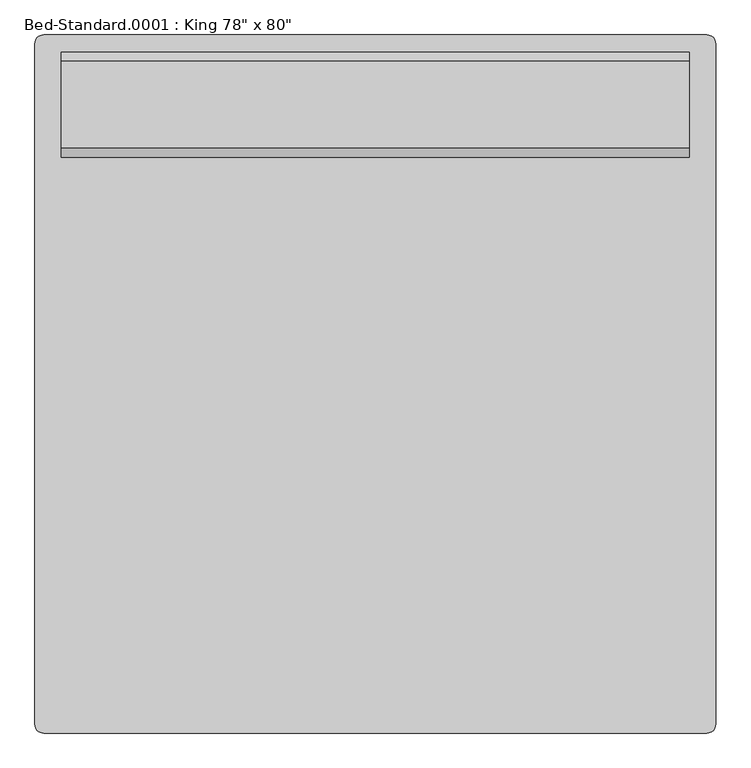
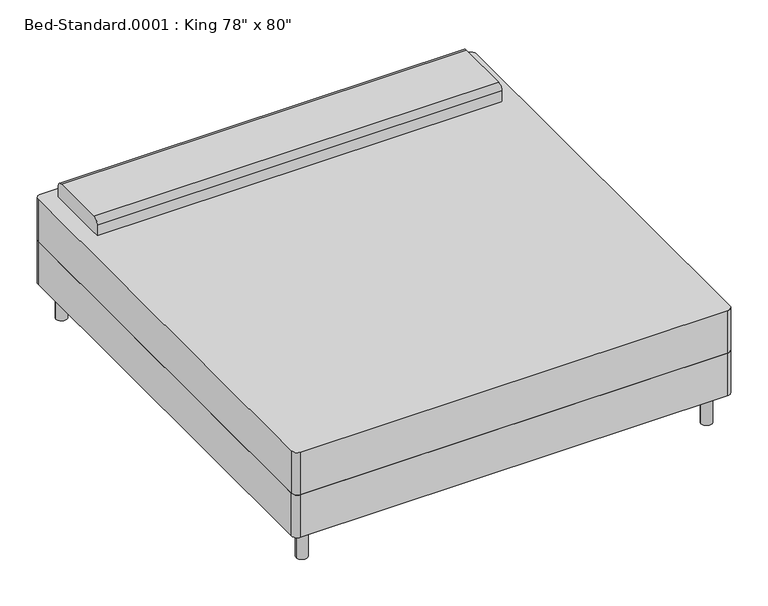
"""IFC4 building model written with IfcOpenShell, lengths in millimetres: furniture geometry."""

from ifc_helpers import new_model, si_unit, point, frame, frame_2d, origin, origin_with_axes, place, context, project, spatial, polyline, circle_curve, trimmed, segment, composite_curve, outline, extrude, source, transform, mapped, element, save


def furniture_1fc5af50(model_context):
    return source(origin(), model_context, "Body", "SweptSolid", [
        extrude(outline(composite_curve([segment(polyline([(-719.1114754, -1036.195082), (-719.1114754, 945.004918)]), True, "CONTINUOUS"), segment(trimmed(circle_curve(frame_2d((-693.7114754, 945.004918)), 25.4), [point((-719.1114754, 945.004918))], [point((-693.7114754, 970.404918))], False, "CARTESIAN"), True, "CONTINUOUS"), segment(polyline([(-693.7114754, 970.404918), (1236.6885246, 970.404918)]), True, "CONTINUOUS"), segment(trimmed(circle_curve(frame_2d((1236.6885246, 945.004918)), 25.4), [point((1236.6885246, 970.404918))], [point((1262.0885246, 945.004918))], False, "CARTESIAN"), True, "CONTINUOUS"), segment(polyline([(1262.0885246, 945.004918), (1262.0885246, -1036.195082)]), True, "CONTINUOUS"), segment(trimmed(circle_curve(frame_2d((1236.6885246, -1036.195082)), 25.4), [point((1262.0885246, -1036.195082))], [point((1236.6885246, -1061.595082))], False, "CARTESIAN"), True, "CONTINUOUS"), segment(polyline([(1236.6885246, -1061.595082), (-693.7114754, -1061.595082)]), True, "CONTINUOUS"), segment(trimmed(circle_curve(frame_2d((-693.7114754, -1036.195082)), 25.4), [point((-693.7114754, -1061.595082))], [point((-719.1114754, -1036.195082))], False, "CARTESIAN"), True, "CONTINUOUS")], self_intersect=False)), frame((0.0, 0.0, 152.4), z_axis=(0.0, 0.0, 1.0), x_axis=(1.0, 0.0, 0.0)), (0.0, 0.0, 1.0), 203.2),
        extrude(outline(composite_curve([segment(polyline([(614.804918, 558.8), (614.804918, 609.6)]), True, "CONTINUOUS"), segment(trimmed(circle_curve(frame_2d((640.204918, 609.6)), 25.4), [point((614.804918, 609.6))], [point((640.204918, 635.0))], False, "CARTESIAN"), True, "CONTINUOUS"), segment(polyline([(640.204918, 635.0), (894.204918, 635.0)]), True, "CONTINUOUS"), segment(trimmed(circle_curve(frame_2d((894.204918, 609.6)), 25.4), [point((894.204918, 635.0))], [point((919.604918, 609.6))], False, "CARTESIAN"), True, "CONTINUOUS"), segment(polyline([(919.604918, 609.6), (919.604918, 558.8), (614.804918, 558.8)]), True, "CONTINUOUS")], self_intersect=False)), frame((-642.9114754, 0.0, 0.0), z_axis=(1.0, 0.0, 0.0), x_axis=(0.0, 1.0, 0.0)), (0.0, 0.0, 1.0), 1828.8),
        extrude(outline(composite_curve([segment(trimmed(circle_curve(frame_2d((-642.9114754, 894.204918)), 25.4), [point((-668.3114754, 894.204918))], [point((-617.5114754, 894.204918))], False, "CARTESIAN"), True, "CONTINUOUS"), segment(trimmed(circle_curve(frame_2d((-642.9114754, 894.204918)), 25.4), [point((-617.5114754, 894.204918))], [point((-668.3114754, 894.204918))], False, "CARTESIAN"), True, "CONTINUOUS")], self_intersect=False)), origin_with_axes(), (0.0, 0.0, 1.0), 152.4),
        extrude(outline(composite_curve([segment(trimmed(circle_curve(frame_2d((1185.8885246, 894.204918)), 25.4), [point((1160.4885246, 894.204918))], [point((1211.2885246, 894.204918))], False, "CARTESIAN"), True, "CONTINUOUS"), segment(trimmed(circle_curve(frame_2d((1185.8885246, 894.204918)), 25.4), [point((1211.2885246, 894.204918))], [point((1160.4885246, 894.204918))], False, "CARTESIAN"), True, "CONTINUOUS")], self_intersect=False)), origin_with_axes(), (0.0, 0.0, 1.0), 152.4),
        extrude(outline(composite_curve([segment(trimmed(circle_curve(frame_2d((1185.8885246, -985.395082)), 25.4), [point((1160.4885246, -985.395082))], [point((1211.2885246, -985.395082))], False, "CARTESIAN"), True, "CONTINUOUS"), segment(trimmed(circle_curve(frame_2d((1185.8885246, -985.395082)), 25.4), [point((1211.2885246, -985.395082))], [point((1160.4885246, -985.395082))], False, "CARTESIAN"), True, "CONTINUOUS")], self_intersect=False)), origin_with_axes(), (0.0, 0.0, 1.0), 152.4),
        extrude(outline(composite_curve([segment(trimmed(circle_curve(frame_2d((-642.9114754, -985.395082)), 25.4), [point((-668.3114754, -985.395082))], [point((-617.5114754, -985.395082))], False, "CARTESIAN"), True, "CONTINUOUS"), segment(trimmed(circle_curve(frame_2d((-642.9114754, -985.395082)), 25.4), [point((-617.5114754, -985.395082))], [point((-668.3114754, -985.395082))], False, "CARTESIAN"), True, "CONTINUOUS")], self_intersect=False)), origin_with_axes(), (0.0, 0.0, 1.0), 152.4),
        extrude(outline(composite_curve([segment(polyline([(-693.7114754, 970.404918), (1236.6885246, 970.404918)]), True, "CONTINUOUS"), segment(trimmed(circle_curve(frame_2d((1236.6885246, 945.004918)), 25.4), [point((1236.6885246, 970.404918))], [point((1262.0885246, 945.004918))], False, "CARTESIAN"), True, "CONTINUOUS"), segment(polyline([(1262.0885246, 945.004918), (1262.0885246, -1036.195082)]), True, "CONTINUOUS"), segment(trimmed(circle_curve(frame_2d((1236.6885246, -1036.195082)), 25.4), [point((1262.0885246, -1036.195082))], [point((1236.6885246, -1061.595082))], False, "CARTESIAN"), True, "CONTINUOUS"), segment(polyline([(1236.6885246, -1061.595082), (-693.7114754, -1061.595082)]), True, "CONTINUOUS"), segment(trimmed(circle_curve(frame_2d((-693.7114754, -1036.195082)), 25.4), [point((-693.7114754, -1061.595082))], [point((-719.1114754, -1036.195082))], False, "CARTESIAN"), True, "CONTINUOUS"), segment(polyline([(-719.1114754, -1036.195082), (-719.1114754, 945.004918)]), True, "CONTINUOUS"), segment(trimmed(circle_curve(frame_2d((-693.7114754, 945.004918)), 25.4), [point((-719.1114754, 945.004918))], [point((-693.7114754, 970.404918))], False, "CARTESIAN"), True, "CONTINUOUS")], self_intersect=False)), frame((0.0, 0.0, 355.6), z_axis=(0.0, 0.0, 1.0), x_axis=(1.0, 0.0, 0.0)), (0.0, 0.0, 1.0), 203.2),
    ])


if __name__ == "__main__":
    model = new_model("IFC4")
    model_context = context("Model", 3, world=origin())
    ifc_project = project(units=[si_unit("LENGTHUNIT", "METRE", prefix="MILLI")], contexts=[model_context])
    site = spatial("IfcSite", under=ifc_project)
    building = spatial("IfcBuilding", under=site)
    placement = place(None, origin())
    furniture_shape = furniture_1fc5af50(model_context)
    element("IfcFurniture", 1, ObjectType="Bed-Standard.0001 : King 78\" x 80\"", at=placement, inside=building, context=model_context, shape_type="MappedRepresentation", body=[
        mapped(furniture_shape, transform((0.0, 0.0, 0.0), x_axis=(1.0, 0.0, 0.0), y_axis=(0.0, 1.0, 0.0), z_axis=(0.0, 0.0, 1.0))),
    ])
    save(model, "model.ifc")

# Revit data of these elements
# Type "Bed-Standard.0001 : King 78\" x 80\""
#   Assembly Code = "E2020200"
#   Length = 6' - 8"
#   Width = 6' - 6"
#   Leg Material = Steel, Chrome Plated
#   Mattress Material = Linen, Beige
#   Default Elevation = 0
# Element 1 (IfcFurniture, "Bed-Standard.0001 : King 78\" x 80\"")
#   Materials on its faces: "Linen, White", "Steel, Chrome Plated"
# Materials
#   "Steel, Chrome Plated": class "Metal", colour RGB 17 17 17, transparency 0, Description = "Chromiuim plated steel", Cost = 0
#   "Linen, Beige": class "Textile", colour RGB 249 239 230, transparency 0, Description = "Linen, beige", Cost = 0
#   "Linen, White": class "Textile", colour RGB 247 247 239, transparency 0, Description = "Linen, white", Cost = 0
